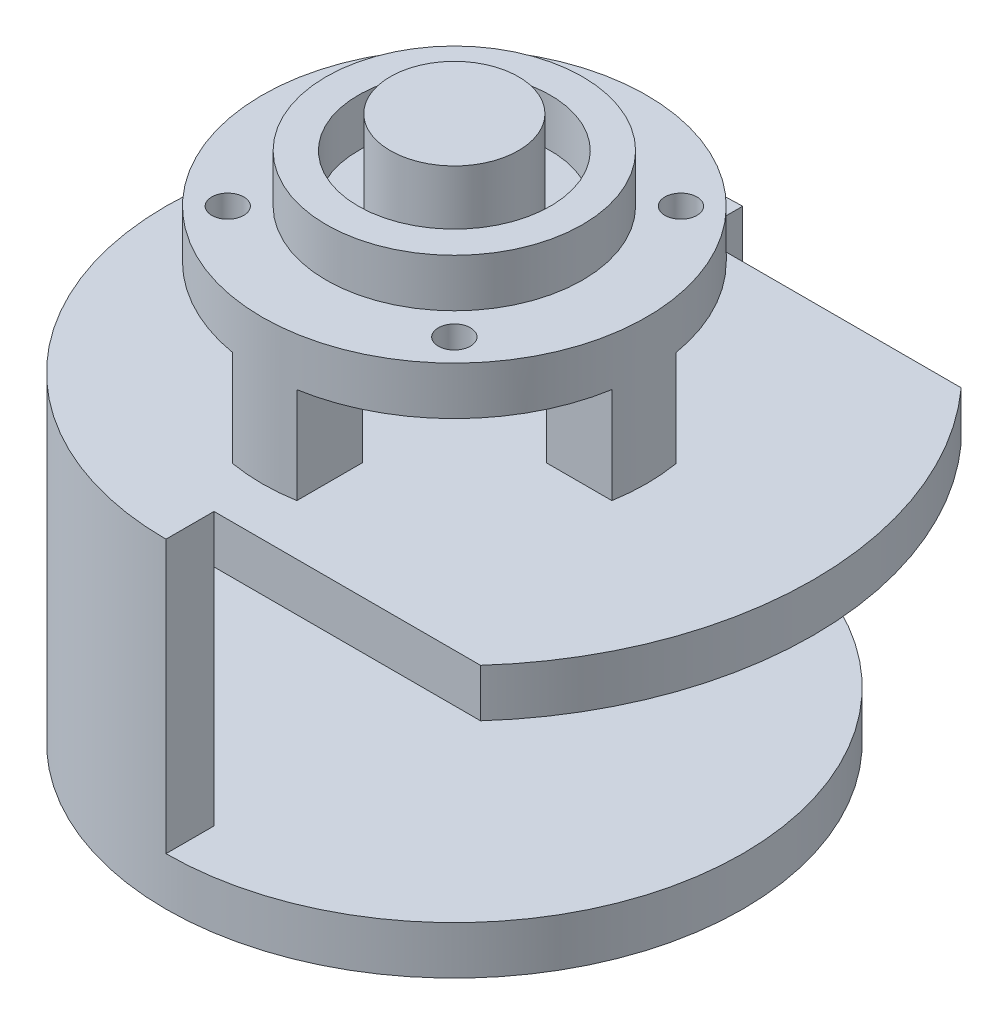
ISO-10303-21;
HEADER;
FILE_DESCRIPTION(('STEP AP214'),'2;1');
FILE_NAME('part.step','',(''),(''),'','','');
FILE_SCHEMA(('AUTOMOTIVE_DESIGN { 1 0 10303 214 1 1 1 1 }'));
ENDSEC;
DATA;
#1=APPLICATION_CONTEXT('core data for automotive mechanical design processes');
#2=APPLICATION_PROTOCOL_DEFINITION('international standard','automotive_design',2000,#1);
#3=PRODUCT_CONTEXT('',#1,'mechanical');
#4=PRODUCT('Part','Part','',(#3));
#5=PRODUCT_RELATED_PRODUCT_CATEGORY('part','',(#4));
#6=PRODUCT_DEFINITION_FORMATION('','',#4);
#7=PRODUCT_DEFINITION_CONTEXT('part definition',#1,'design');
#8=PRODUCT_DEFINITION('design','',#6,#7);
#9=PRODUCT_DEFINITION_SHAPE('','',#8);
#10=(LENGTH_UNIT() NAMED_UNIT(*) SI_UNIT(.MILLI.,.METRE.));
#11=(NAMED_UNIT(*) PLANE_ANGLE_UNIT() SI_UNIT($,.RADIAN.));
#12=(NAMED_UNIT(*) SI_UNIT($,.STERADIAN.) SOLID_ANGLE_UNIT());
#13=UNCERTAINTY_MEASURE_WITH_UNIT(LENGTH_MEASURE(1.E-05),#10,'distance_accuracy_value','');
#14=(GEOMETRIC_REPRESENTATION_CONTEXT(3) GLOBAL_UNCERTAINTY_ASSIGNED_CONTEXT((#13)) GLOBAL_UNIT_ASSIGNED_CONTEXT((#10,
#11,#12)) REPRESENTATION_CONTEXT('',''));
#15=CARTESIAN_POINT('',(0.,0.,0.));
#16=DIRECTION('',(0.,0.,1.));
#17=DIRECTION('',(1.,0.,0.));
#18=AXIS2_PLACEMENT_3D('',#15,#16,#17);
#19=CARTESIAN_POINT('',(0.,15.,0.));
#20=DIRECTION('',(0.,-1.,0.));
#21=DIRECTION('',(0.,0.,-1.));
#22=AXIS2_PLACEMENT_3D('',#19,#20,#21);
#23=CYLINDRICAL_SURFACE('',#22,90.);
#24=CARTESIAN_POINT('',(0.,15.,0.));
#25=DIRECTION('',(0.,1.,0.));
#26=DIRECTION('',(0.,0.,1.));
#27=AXIS2_PLACEMENT_3D('',#24,#25,#26);
#28=CIRCLE('',#27,90.);
#29=CARTESIAN_POINT('',(0.,15.,90.));
#30=VERTEX_POINT('',#29);
#31=CARTESIAN_POINT('',(0.,15.,-90.));
#32=VERTEX_POINT('',#31);
#33=EDGE_CURVE('E297',#30,#32,#28,.T.);
#34=ORIENTED_EDGE('',*,*,#33,.F.);
#35=DIRECTION('',(0.,-1.,0.));
#36=VECTOR('',#35,1.);
#37=CARTESIAN_POINT('',(0.,85.,90.));
#38=LINE('',#37,#36);
#39=CARTESIAN_POINT('',(0.,100.,90.));
#40=VERTEX_POINT('',#39);
#41=EDGE_CURVE('E298',#40,#30,#38,.T.);
#42=ORIENTED_EDGE('',*,*,#41,.F.);
#43=CARTESIAN_POINT('',(0.,100.,0.));
#44=DIRECTION('',(0.,1.,0.));
#45=DIRECTION('',(0.,0.,1.));
#46=AXIS2_PLACEMENT_3D('',#43,#44,#45);
#47=CIRCLE('',#46,90.);
#48=CARTESIAN_POINT('',(0.,100.,-90.));
#49=VERTEX_POINT('',#48);
#50=EDGE_CURVE('E242',#49,#40,#47,.T.);
#51=ORIENTED_EDGE('',*,*,#50,.F.);
#52=DIRECTION('',(0.,-1.,0.));
#53=VECTOR('',#52,1.);
#54=CARTESIAN_POINT('',(0.,85.,-90.));
#55=LINE('',#54,#53);
#56=EDGE_CURVE('E276',#49,#32,#55,.T.);
#57=ORIENTED_EDGE('',*,*,#56,.T.);
#58=EDGE_LOOP('',(#34,#42,#51,#57));
#59=FACE_BOUND('',#58,.T.);
#60=CARTESIAN_POINT('',(0.,0.,0.));
#61=DIRECTION('',(0.,1.,0.));
#62=DIRECTION('',(0.,0.,1.));
#63=AXIS2_PLACEMENT_3D('',#60,#61,#62);
#64=CIRCLE('',#63,90.);
#65=CARTESIAN_POINT('',(0.,0.,90.));
#66=VERTEX_POINT('',#65);
#67=EDGE_CURVE('E299',#66,#66,#64,.T.);
#68=ORIENTED_EDGE('',*,*,#67,.T.);
#69=EDGE_LOOP('',(#68));
#70=FACE_BOUND('',#69,.T.);
#71=ADVANCED_FACE('F50',(#59,#70),#23,.T.);
#72=CARTESIAN_POINT('',(0.,15.,0.));
#73=DIRECTION('',(0.,1.,0.));
#74=DIRECTION('',(0.,0.,1.));
#75=AXIS2_PLACEMENT_3D('',#72,#73,#74);
#76=PLANE('',#75);
#77=DIRECTION('',(0.,0.,-1.));
#78=VECTOR('',#77,1.);
#79=CARTESIAN_POINT('',(0.,15.,-75.));
#80=LINE('',#79,#78);
#81=CARTESIAN_POINT('',(0.,15.,-75.));
#82=VERTEX_POINT('',#81);
#83=EDGE_CURVE('E278',#82,#32,#80,.T.);
#84=ORIENTED_EDGE('',*,*,#83,.F.);
#85=CARTESIAN_POINT('',(0.,15.,0.));
#86=DIRECTION('',(0.,-1.,0.));
#87=DIRECTION('',(0.,0.,1.));
#88=AXIS2_PLACEMENT_3D('',#85,#86,#87);
#89=CIRCLE('',#88,75.);
#90=CARTESIAN_POINT('',(0.,15.,75.));
#91=VERTEX_POINT('',#90);
#92=EDGE_CURVE('E281',#91,#82,#89,.T.);
#93=ORIENTED_EDGE('',*,*,#92,.F.);
#94=DIRECTION('',(0.,0.,-1.));
#95=VECTOR('',#94,1.);
#96=CARTESIAN_POINT('',(0.,15.,90.));
#97=LINE('',#96,#95);
#98=EDGE_CURVE('E274',#30,#91,#97,.T.);
#99=ORIENTED_EDGE('',*,*,#98,.F.);
#100=ORIENTED_EDGE('',*,*,#33,.T.);
#101=EDGE_LOOP('',(#84,#93,#99,#100));
#102=FACE_BOUND('',#101,.T.);
#103=ADVANCED_FACE('F437',(#102),#76,.T.);
#104=CARTESIAN_POINT('',(0.,0.,0.));
#105=DIRECTION('',(0.,1.,0.));
#106=DIRECTION('',(0.,0.,1.));
#107=AXIS2_PLACEMENT_3D('',#104,#105,#106);
#108=PLANE('',#107);
#109=ORIENTED_EDGE('',*,*,#67,.F.);
#110=EDGE_LOOP('',(#109));
#111=FACE_BOUND('',#110,.T.);
#112=ADVANCED_FACE('F443',(#111),#108,.F.);
#113=CARTESIAN_POINT('',(0.,85.,90.));
#114=DIRECTION('',(-1.,0.,0.));
#115=DIRECTION('',(0.,0.,1.));
#116=AXIS2_PLACEMENT_3D('',#113,#114,#115);
#117=PLANE('',#116);
#118=ORIENTED_EDGE('',*,*,#98,.T.);
#119=DIRECTION('',(0.,-1.,0.));
#120=VECTOR('',#119,1.);
#121=CARTESIAN_POINT('',(0.,85.,75.));
#122=LINE('',#121,#120);
#123=CARTESIAN_POINT('',(0.,85.,75.));
#124=VERTEX_POINT('',#123);
#125=EDGE_CURVE('E291',#124,#91,#122,.T.);
#126=ORIENTED_EDGE('',*,*,#125,.F.);
#127=DIRECTION('',(0.,-1.,0.));
#128=VECTOR('',#127,1.);
#129=CARTESIAN_POINT('',(0.,100.,75.));
#130=LINE('',#129,#128);
#131=CARTESIAN_POINT('',(0.,100.,75.));
#132=VERTEX_POINT('',#131);
#133=EDGE_CURVE('E275',#132,#124,#130,.T.);
#134=ORIENTED_EDGE('',*,*,#133,.F.);
#135=DIRECTION('',(0.,0.,-1.));
#136=VECTOR('',#135,1.);
#137=CARTESIAN_POINT('',(0.,100.,0.));
#138=LINE('',#137,#136);
#139=EDGE_CURVE('E248',#40,#132,#138,.T.);
#140=ORIENTED_EDGE('',*,*,#139,.F.);
#141=ORIENTED_EDGE('',*,*,#41,.T.);
#142=EDGE_LOOP('',(#118,#126,#134,#140,#141));
#143=FACE_BOUND('',#142,.T.);
#144=ADVANCED_FACE('F454',(#143),#117,.F.);
#145=CARTESIAN_POINT('',(0.,85.,0.));
#146=DIRECTION('',(0.,-1.,0.));
#147=DIRECTION('',(0.,0.,-1.));
#148=AXIS2_PLACEMENT_3D('',#145,#146,#147);
#149=CYLINDRICAL_SURFACE('',#148,75.);
#150=ORIENTED_EDGE('',*,*,#92,.T.);
#151=DIRECTION('',(0.,-1.,0.));
#152=VECTOR('',#151,1.);
#153=CARTESIAN_POINT('',(0.,85.,-75.));
#154=LINE('',#153,#152);
#155=CARTESIAN_POINT('',(0.,85.,-75.));
#156=VERTEX_POINT('',#155);
#157=EDGE_CURVE('E290',#156,#82,#154,.T.);
#158=ORIENTED_EDGE('',*,*,#157,.F.);
#159=CARTESIAN_POINT('',(0.,85.,0.));
#160=DIRECTION('',(0.,-1.,0.));
#161=DIRECTION('',(0.,0.,1.));
#162=AXIS2_PLACEMENT_3D('',#159,#160,#161);
#163=CIRCLE('',#162,75.);
#164=EDGE_CURVE('E277',#124,#156,#163,.T.);
#165=ORIENTED_EDGE('',*,*,#164,.F.);
#166=ORIENTED_EDGE('',*,*,#125,.T.);
#167=EDGE_LOOP('',(#150,#158,#165,#166));
#168=FACE_BOUND('',#167,.T.);
#169=ADVANCED_FACE('F457',(#168),#149,.F.);
#170=CARTESIAN_POINT('',(0.,85.,-75.));
#171=DIRECTION('',(-1.,0.,0.));
#172=DIRECTION('',(0.,0.,1.));
#173=AXIS2_PLACEMENT_3D('',#170,#171,#172);
#174=PLANE('',#173);
#175=ORIENTED_EDGE('',*,*,#83,.T.);
#176=ORIENTED_EDGE('',*,*,#56,.F.);
#177=DIRECTION('',(0.,0.,-1.));
#178=VECTOR('',#177,1.);
#179=CARTESIAN_POINT('',(0.,100.,0.));
#180=LINE('',#179,#178);
#181=CARTESIAN_POINT('',(0.,100.,-75.));
#182=VERTEX_POINT('',#181);
#183=EDGE_CURVE('E245',#182,#49,#180,.T.);
#184=ORIENTED_EDGE('',*,*,#183,.F.);
#185=DIRECTION('',(0.,-1.,0.));
#186=VECTOR('',#185,1.);
#187=CARTESIAN_POINT('',(0.,100.,-75.));
#188=LINE('',#187,#186);
#189=EDGE_CURVE('E256',#182,#156,#188,.T.);
#190=ORIENTED_EDGE('',*,*,#189,.T.);
#191=ORIENTED_EDGE('',*,*,#157,.T.);
#192=EDGE_LOOP('',(#175,#176,#184,#190,#191));
#193=FACE_BOUND('',#192,.T.);
#194=ADVANCED_FACE('F465',(#193),#174,.F.);
#195=CARTESIAN_POINT('',(0.,85.,0.));
#196=DIRECTION('',(0.,1.,0.));
#197=DIRECTION('',(0.,0.,1.));
#198=AXIS2_PLACEMENT_3D('',#195,#196,#197);
#199=PLANE('',#198);
#200=DIRECTION('',(1.,0.,0.));
#201=VECTOR('',#200,1.);
#202=CARTESIAN_POINT('',(0.,85.,75.));
#203=LINE('',#202,#201);
#204=CARTESIAN_POINT('',(83.18052656722,85.,75.));
#205=VERTEX_POINT('',#204);
#206=EDGE_CURVE('E233',#124,#205,#203,.T.);
#207=ORIENTED_EDGE('',*,*,#206,.F.);
#208=ORIENTED_EDGE('',*,*,#164,.T.);
#209=DIRECTION('',(1.,0.,0.));
#210=VECTOR('',#209,1.);
#211=CARTESIAN_POINT('',(0.,85.,-75.));
#212=LINE('',#211,#210);
#213=CARTESIAN_POINT('',(83.18052656722,85.,-75.));
#214=VERTEX_POINT('',#213);
#215=EDGE_CURVE('E246',#156,#214,#212,.T.);
#216=ORIENTED_EDGE('',*,*,#215,.T.);
#217=CARTESIAN_POINT('',(0.,85.,0.));
#218=DIRECTION('',(0.,1.,0.));
#219=DIRECTION('',(0.,0.,1.));
#220=AXIS2_PLACEMENT_3D('',#217,#218,#219);
#221=CIRCLE('',#220,112.);
#222=EDGE_CURVE('E257',#205,#214,#221,.T.);
#223=ORIENTED_EDGE('',*,*,#222,.F.);
#224=EDGE_LOOP('',(#207,#208,#216,#223));
#225=FACE_BOUND('',#224,.T.);
#226=ADVANCED_FACE('F466',(#225),#199,.F.);
#227=CARTESIAN_POINT('',(0.,100.,75.));
#228=DIRECTION('',(0.,0.,-1.));
#229=DIRECTION('',(-1.,0.,0.));
#230=AXIS2_PLACEMENT_3D('',#227,#228,#229);
#231=PLANE('',#230);
#232=ORIENTED_EDGE('',*,*,#206,.T.);
#233=DIRECTION('',(0.,-1.,0.));
#234=VECTOR('',#233,1.);
#235=CARTESIAN_POINT('',(83.18052656722,100.,75.));
#236=LINE('',#235,#234);
#237=CARTESIAN_POINT('',(83.18052656722,100.,75.));
#238=VERTEX_POINT('',#237);
#239=EDGE_CURVE('E267',#238,#205,#236,.T.);
#240=ORIENTED_EDGE('',*,*,#239,.F.);
#241=DIRECTION('',(1.,0.,0.));
#242=VECTOR('',#241,1.);
#243=CARTESIAN_POINT('',(0.,100.,75.));
#244=LINE('',#243,#242);
#245=EDGE_CURVE('E253',#132,#238,#244,.T.);
#246=ORIENTED_EDGE('',*,*,#245,.F.);
#247=ORIENTED_EDGE('',*,*,#133,.T.);
#248=EDGE_LOOP('',(#232,#240,#246,#247));
#249=FACE_BOUND('',#248,.T.);
#250=ADVANCED_FACE('F469',(#249),#231,.F.);
#251=CARTESIAN_POINT('',(0.,100.,0.));
#252=DIRECTION('',(0.,-1.,0.));
#253=DIRECTION('',(0.,0.,-1.));
#254=AXIS2_PLACEMENT_3D('',#251,#252,#253);
#255=CYLINDRICAL_SURFACE('',#254,112.);
#256=ORIENTED_EDGE('',*,*,#222,.T.);
#257=DIRECTION('',(0.,-1.,0.));
#258=VECTOR('',#257,1.);
#259=CARTESIAN_POINT('',(83.18052656722,100.,-75.));
#260=LINE('',#259,#258);
#261=CARTESIAN_POINT('',(83.18052656722,100.,-75.));
#262=VERTEX_POINT('',#261);
#263=EDGE_CURVE('E270',#262,#214,#260,.T.);
#264=ORIENTED_EDGE('',*,*,#263,.F.);
#265=CARTESIAN_POINT('',(0.,100.,0.));
#266=DIRECTION('',(0.,1.,0.));
#267=DIRECTION('',(0.,0.,1.));
#268=AXIS2_PLACEMENT_3D('',#265,#266,#267);
#269=CIRCLE('',#268,112.);
#270=EDGE_CURVE('E251',#238,#262,#269,.T.);
#271=ORIENTED_EDGE('',*,*,#270,.F.);
#272=ORIENTED_EDGE('',*,*,#239,.T.);
#273=EDGE_LOOP('',(#256,#264,#271,#272));
#274=FACE_BOUND('',#273,.T.);
#275=ADVANCED_FACE('F473',(#274),#255,.T.);
#276=CARTESIAN_POINT('',(0.,100.,-75.));
#277=DIRECTION('',(0.,0.,-1.));
#278=DIRECTION('',(-1.,0.,0.));
#279=AXIS2_PLACEMENT_3D('',#276,#277,#278);
#280=PLANE('',#279);
#281=ORIENTED_EDGE('',*,*,#215,.F.);
#282=ORIENTED_EDGE('',*,*,#189,.F.);
#283=DIRECTION('',(1.,0.,0.));
#284=VECTOR('',#283,1.);
#285=CARTESIAN_POINT('',(0.,100.,-75.));
#286=LINE('',#285,#284);
#287=EDGE_CURVE('E254',#182,#262,#286,.T.);
#288=ORIENTED_EDGE('',*,*,#287,.T.);
#289=ORIENTED_EDGE('',*,*,#263,.T.);
#290=EDGE_LOOP('',(#281,#282,#288,#289));
#291=FACE_BOUND('',#290,.T.);
#292=ADVANCED_FACE('F474',(#291),#280,.T.);
#293=CARTESIAN_POINT('',(0.,100.,0.));
#294=DIRECTION('',(0.,1.,0.));
#295=DIRECTION('',(0.,0.,1.));
#296=AXIS2_PLACEMENT_3D('',#293,#294,#295);
#297=PLANE('',#296);
#298=CARTESIAN_POINT('',(0.,100.,0.));
#299=DIRECTION('',(0.,1.,0.));
#300=DIRECTION('',(0.,0.,1.));
#301=AXIS2_PLACEMENT_3D('',#298,#299,#300);
#302=CIRCLE('',#301,60.);
#303=CARTESIAN_POINT('',(-10.,100.,59.1607978309962));
#304=VERTEX_POINT('',#303);
#305=CARTESIAN_POINT('',(9.99999999999999,100.,59.1607978309962));
#306=VERTEX_POINT('',#305);
#307=EDGE_CURVE('E235',#304,#306,#302,.T.);
#308=ORIENTED_EDGE('',*,*,#307,.F.);
#309=DIRECTION('',(0.,0.,-1.));
#310=VECTOR('',#309,1.);
#311=CARTESIAN_POINT('',(-10.,100.,59.1607978309962));
#312=LINE('',#311,#310);
#313=CARTESIAN_POINT('',(-10.,100.,38.7298334620742));
#314=VERTEX_POINT('',#313);
#315=EDGE_CURVE('E380',#304,#314,#312,.T.);
#316=ORIENTED_EDGE('',*,*,#315,.T.);
#317=CARTESIAN_POINT('',(0.,100.,0.));
#318=DIRECTION('',(0.,1.,0.));
#319=DIRECTION('',(0.,0.,1.));
#320=AXIS2_PLACEMENT_3D('',#317,#318,#319);
#321=CIRCLE('',#320,40.);
#322=CARTESIAN_POINT('',(9.99999999999998,100.,38.7298334620742));
#323=VERTEX_POINT('',#322);
#324=EDGE_CURVE('E302',#323,#314,#321,.F.);
#325=ORIENTED_EDGE('',*,*,#324,.F.);
#326=DIRECTION('',(0.,0.,1.));
#327=VECTOR('',#326,1.);
#328=CARTESIAN_POINT('',(9.99999999999999,100.,59.1607978309962));
#329=LINE('',#328,#327);
#330=EDGE_CURVE('E392',#323,#306,#329,.T.);
#331=ORIENTED_EDGE('',*,*,#330,.T.);
#332=EDGE_LOOP('',(#308,#316,#325,#331));
#333=FACE_BOUND('',#332,.T.);
#334=CARTESIAN_POINT('',(59.1607978309962,100.,10.));
#335=VERTEX_POINT('',#334);
#336=CARTESIAN_POINT('',(59.1607978309962,100.,-9.99999999999998));
#337=VERTEX_POINT('',#336);
#338=EDGE_CURVE('E227',#335,#337,#302,.T.);
#339=ORIENTED_EDGE('',*,*,#338,.F.);
#340=DIRECTION('',(-1.,0.,0.));
#341=VECTOR('',#340,1.);
#342=CARTESIAN_POINT('',(59.1607978309962,100.,10.));
#343=LINE('',#342,#341);
#344=CARTESIAN_POINT('',(38.7298334620742,100.,10.));
#345=VERTEX_POINT('',#344);
#346=EDGE_CURVE('E399',#335,#345,#343,.T.);
#347=ORIENTED_EDGE('',*,*,#346,.T.);
#348=CARTESIAN_POINT('',(38.7298334620742,100.,-9.99999999999998));
#349=VERTEX_POINT('',#348);
#350=EDGE_CURVE('E305',#349,#345,#321,.F.);
#351=ORIENTED_EDGE('',*,*,#350,.F.);
#352=DIRECTION('',(1.,0.,0.));
#353=VECTOR('',#352,1.);
#354=CARTESIAN_POINT('',(59.1607978309962,100.,-9.99999999999998));
#355=LINE('',#354,#353);
#356=EDGE_CURVE('E213',#349,#337,#355,.T.);
#357=ORIENTED_EDGE('',*,*,#356,.T.);
#358=EDGE_LOOP('',(#339,#347,#351,#357));
#359=FACE_BOUND('',#358,.T.);
#360=CARTESIAN_POINT('',(10.,100.,-59.1607978309962));
#361=VERTEX_POINT('',#360);
#362=CARTESIAN_POINT('',(-10.,100.,-59.1607978309962));
#363=VERTEX_POINT('',#362);
#364=EDGE_CURVE('E225',#361,#363,#302,.T.);
#365=ORIENTED_EDGE('',*,*,#364,.F.);
#366=DIRECTION('',(0.,0.,1.));
#367=VECTOR('',#366,1.);
#368=CARTESIAN_POINT('',(10.,100.,-59.1607978309962));
#369=LINE('',#368,#367);
#370=CARTESIAN_POINT('',(10.,100.,-38.7298334620742));
#371=VERTEX_POINT('',#370);
#372=EDGE_CURVE('E203',#361,#371,#369,.T.);
#373=ORIENTED_EDGE('',*,*,#372,.T.);
#374=CARTESIAN_POINT('',(-10.,100.,-38.7298334620742));
#375=VERTEX_POINT('',#374);
#376=EDGE_CURVE('E313',#375,#371,#321,.F.);
#377=ORIENTED_EDGE('',*,*,#376,.F.);
#378=DIRECTION('',(0.,0.,-1.));
#379=VECTOR('',#378,1.);
#380=CARTESIAN_POINT('',(-10.,100.,-59.1607978309962));
#381=LINE('',#380,#379);
#382=EDGE_CURVE('E229',#375,#363,#381,.T.);
#383=ORIENTED_EDGE('',*,*,#382,.T.);
#384=EDGE_LOOP('',(#365,#373,#377,#383));
#385=FACE_BOUND('',#384,.T.);
#386=DIRECTION('',(-1.,0.,0.));
#387=VECTOR('',#386,1.);
#388=CARTESIAN_POINT('',(-59.1607978309962,100.,9.99999999999999));
#389=LINE('',#388,#387);
#390=CARTESIAN_POINT('',(-38.7298334620742,100.,9.99999999999997));
#391=VERTEX_POINT('',#390);
#392=CARTESIAN_POINT('',(-59.1607978309962,100.,9.99999999999999));
#393=VERTEX_POINT('',#392);
#394=EDGE_CURVE('E356',#391,#393,#389,.T.);
#395=ORIENTED_EDGE('',*,*,#394,.T.);
#396=CARTESIAN_POINT('',(-59.1607978309962,100.,-10.));
#397=VERTEX_POINT('',#396);
#398=EDGE_CURVE('E231',#397,#393,#302,.T.);
#399=ORIENTED_EDGE('',*,*,#398,.F.);
#400=DIRECTION('',(1.,0.,0.));
#401=VECTOR('',#400,1.);
#402=CARTESIAN_POINT('',(-59.1607978309962,100.,-10.));
#403=LINE('',#402,#401);
#404=CARTESIAN_POINT('',(-38.7298334620742,100.,-10.));
#405=VERTEX_POINT('',#404);
#406=EDGE_CURVE('E340',#397,#405,#403,.T.);
#407=ORIENTED_EDGE('',*,*,#406,.T.);
#408=EDGE_CURVE('E53',#391,#405,#321,.F.);
#409=ORIENTED_EDGE('',*,*,#408,.F.);
#410=EDGE_LOOP('',(#395,#399,#407,#409));
#411=FACE_BOUND('',#410,.T.);
#412=ORIENTED_EDGE('',*,*,#183,.T.);
#413=ORIENTED_EDGE('',*,*,#50,.T.);
#414=ORIENTED_EDGE('',*,*,#139,.T.);
#415=ORIENTED_EDGE('',*,*,#245,.T.);
#416=ORIENTED_EDGE('',*,*,#270,.T.);
#417=ORIENTED_EDGE('',*,*,#287,.F.);
#418=EDGE_LOOP('',(#412,#413,#414,#415,#416,#417));
#419=FACE_BOUND('',#418,.T.);
#420=ADVANCED_FACE('F230',(#333,#359,#385,#411,#419),#297,.T.);
#421=CARTESIAN_POINT('',(0.,140.,0.));
#422=DIRECTION('',(0.,-1.,0.));
#423=DIRECTION('',(0.,0.,-1.));
#424=AXIS2_PLACEMENT_3D('',#421,#422,#423);
#425=CYLINDRICAL_SURFACE('',#424,60.);
#426=ORIENTED_EDGE('',*,*,#398,.T.);
#427=DIRECTION('',(0.,1.,0.));
#428=VECTOR('',#427,1.);
#429=CARTESIAN_POINT('',(-59.1607978309962,100.,9.99999999999999));
#430=LINE('',#429,#428);
#431=CARTESIAN_POINT('',(-59.1607978309962,130.,9.99999999999999));
#432=VERTEX_POINT('',#431);
#433=EDGE_CURVE('E358',#393,#432,#430,.T.);
#434=ORIENTED_EDGE('',*,*,#433,.T.);
#435=CARTESIAN_POINT('',(0.,130.,0.));
#436=DIRECTION('',(0.,1.,0.));
#437=DIRECTION('',(0.,0.,1.));
#438=AXIS2_PLACEMENT_3D('',#435,#436,#437);
#439=CIRCLE('',#438,60.);
#440=CARTESIAN_POINT('',(-10.,130.,59.1607978309962));
#441=VERTEX_POINT('',#440);
#442=EDGE_CURVE('E363',#432,#441,#439,.T.);
#443=ORIENTED_EDGE('',*,*,#442,.T.);
#444=DIRECTION('',(0.,1.,0.));
#445=VECTOR('',#444,1.);
#446=CARTESIAN_POINT('',(-10.,100.,59.1607978309962));
#447=LINE('',#446,#445);
#448=EDGE_CURVE('E374',#304,#441,#447,.T.);
#449=ORIENTED_EDGE('',*,*,#448,.F.);
#450=ORIENTED_EDGE('',*,*,#307,.T.);
#451=DIRECTION('',(0.,1.,0.));
#452=VECTOR('',#451,1.);
#453=CARTESIAN_POINT('',(9.99999999999999,100.,59.1607978309962));
#454=LINE('',#453,#452);
#455=CARTESIAN_POINT('',(9.99999999999999,130.,59.1607978309962));
#456=VERTEX_POINT('',#455);
#457=EDGE_CURVE('E407',#306,#456,#454,.T.);
#458=ORIENTED_EDGE('',*,*,#457,.T.);
#459=CARTESIAN_POINT('',(0.,130.,0.));
#460=DIRECTION('',(0.,1.,0.));
#461=DIRECTION('',(0.,0.,1.));
#462=AXIS2_PLACEMENT_3D('',#459,#460,#461);
#463=CIRCLE('',#462,60.);
#464=CARTESIAN_POINT('',(59.1607978309962,130.,10.));
#465=VERTEX_POINT('',#464);
#466=EDGE_CURVE('E365',#456,#465,#463,.T.);
#467=ORIENTED_EDGE('',*,*,#466,.T.);
#468=DIRECTION('',(0.,1.,0.));
#469=VECTOR('',#468,1.);
#470=CARTESIAN_POINT('',(59.1607978309962,100.,10.));
#471=LINE('',#470,#469);
#472=EDGE_CURVE('E397',#335,#465,#471,.T.);
#473=ORIENTED_EDGE('',*,*,#472,.F.);
#474=ORIENTED_EDGE('',*,*,#338,.T.);
#475=DIRECTION('',(0.,1.,0.));
#476=VECTOR('',#475,1.);
#477=CARTESIAN_POINT('',(59.1607978309962,100.,-9.99999999999998));
#478=LINE('',#477,#476);
#479=CARTESIAN_POINT('',(59.1607978309962,130.,-9.99999999999998));
#480=VERTEX_POINT('',#479);
#481=EDGE_CURVE('E347',#337,#480,#478,.T.);
#482=ORIENTED_EDGE('',*,*,#481,.T.);
#483=CARTESIAN_POINT('',(0.,130.,0.));
#484=DIRECTION('',(0.,1.,0.));
#485=DIRECTION('',(0.,0.,1.));
#486=AXIS2_PLACEMENT_3D('',#483,#484,#485);
#487=CIRCLE('',#486,60.);
#488=CARTESIAN_POINT('',(10.,130.,-59.1607978309962));
#489=VERTEX_POINT('',#488);
#490=EDGE_CURVE('E221',#480,#489,#487,.T.);
#491=ORIENTED_EDGE('',*,*,#490,.T.);
#492=DIRECTION('',(0.,1.,0.));
#493=VECTOR('',#492,1.);
#494=CARTESIAN_POINT('',(10.,100.,-59.1607978309962));
#495=LINE('',#494,#493);
#496=EDGE_CURVE('E202',#361,#489,#495,.T.);
#497=ORIENTED_EDGE('',*,*,#496,.F.);
#498=ORIENTED_EDGE('',*,*,#364,.T.);
#499=DIRECTION('',(0.,1.,0.));
#500=VECTOR('',#499,1.);
#501=CARTESIAN_POINT('',(-10.,100.,-59.1607978309962));
#502=LINE('',#501,#500);
#503=CARTESIAN_POINT('',(-10.,130.,-59.1607978309962));
#504=VERTEX_POINT('',#503);
#505=EDGE_CURVE('E239',#363,#504,#502,.T.);
#506=ORIENTED_EDGE('',*,*,#505,.T.);
#507=CARTESIAN_POINT('',(0.,130.,0.));
#508=DIRECTION('',(0.,1.,0.));
#509=DIRECTION('',(0.,0.,1.));
#510=AXIS2_PLACEMENT_3D('',#507,#508,#509);
#511=CIRCLE('',#510,60.);
#512=CARTESIAN_POINT('',(-59.1607978309962,130.,-10.));
#513=VERTEX_POINT('',#512);
#514=EDGE_CURVE('E344',#504,#513,#511,.T.);
#515=ORIENTED_EDGE('',*,*,#514,.T.);
#516=DIRECTION('',(0.,1.,0.));
#517=VECTOR('',#516,1.);
#518=CARTESIAN_POINT('',(-59.1607978309962,100.,-10.));
#519=LINE('',#518,#517);
#520=EDGE_CURVE('E328',#397,#513,#519,.T.);
#521=ORIENTED_EDGE('',*,*,#520,.F.);
#522=EDGE_LOOP('',(#426,#434,#443,#449,#450,#458,#467,#473,#474,#482,#491,#497,#498,#506,#515,#521));
#523=FACE_BOUND('',#522,.T.);
#524=CARTESIAN_POINT('',(0.,145.,0.));
#525=DIRECTION('',(0.,1.,0.));
#526=DIRECTION('',(0.,0.,1.));
#527=AXIS2_PLACEMENT_3D('',#524,#525,#526);
#528=CIRCLE('',#527,60.);
#529=CARTESIAN_POINT('',(0.,145.,60.));
#530=VERTEX_POINT('',#529);
#531=EDGE_CURVE('E517',#530,#530,#528,.T.);
#532=ORIENTED_EDGE('',*,*,#531,.F.);
#533=EDGE_LOOP('',(#532));
#534=FACE_BOUND('',#533,.T.);
#535=ADVANCED_FACE('F218',(#523,#534),#425,.T.);
#536=CARTESIAN_POINT('',(0.,140.,0.));
#537=DIRECTION('',(0.,-1.,0.));
#538=DIRECTION('',(0.,0.,-1.));
#539=AXIS2_PLACEMENT_3D('',#536,#537,#538);
#540=CYLINDRICAL_SURFACE('',#539,40.);
#541=DIRECTION('',(0.,1.,0.));
#542=VECTOR('',#541,1.);
#543=CARTESIAN_POINT('',(-38.7298334620742,100.,9.99999999999997));
#544=LINE('',#543,#542);
#545=CARTESIAN_POINT('',(-38.7298334620742,130.,9.99999999999997));
#546=VERTEX_POINT('',#545);
#547=EDGE_CURVE('E364',#391,#546,#544,.T.);
#548=ORIENTED_EDGE('',*,*,#547,.F.);
#549=ORIENTED_EDGE('',*,*,#408,.T.);
#550=DIRECTION('',(0.,1.,0.));
#551=VECTOR('',#550,1.);
#552=CARTESIAN_POINT('',(-38.7298334620742,100.,-10.));
#553=LINE('',#552,#551);
#554=CARTESIAN_POINT('',(-38.7298334620742,130.,-10.));
#555=VERTEX_POINT('',#554);
#556=EDGE_CURVE('E326',#405,#555,#553,.T.);
#557=ORIENTED_EDGE('',*,*,#556,.T.);
#558=CARTESIAN_POINT('',(0.,130.,0.));
#559=DIRECTION('',(0.,-1.,0.));
#560=DIRECTION('',(0.,0.,1.));
#561=AXIS2_PLACEMENT_3D('',#558,#559,#560);
#562=CIRCLE('',#561,40.);
#563=CARTESIAN_POINT('',(-10.,130.,-38.7298334620742));
#564=VERTEX_POINT('',#563);
#565=EDGE_CURVE('E325',#555,#564,#562,.T.);
#566=ORIENTED_EDGE('',*,*,#565,.T.);
#567=DIRECTION('',(0.,1.,0.));
#568=VECTOR('',#567,1.);
#569=CARTESIAN_POINT('',(-10.,100.,-38.7298334620742));
#570=LINE('',#569,#568);
#571=EDGE_CURVE('E321',#375,#564,#570,.T.);
#572=ORIENTED_EDGE('',*,*,#571,.F.);
#573=ORIENTED_EDGE('',*,*,#376,.T.);
#574=DIRECTION('',(0.,1.,0.));
#575=VECTOR('',#574,1.);
#576=CARTESIAN_POINT('',(10.,100.,-38.7298334620742));
#577=LINE('',#576,#575);
#578=CARTESIAN_POINT('',(10.,130.,-38.7298334620742));
#579=VERTEX_POINT('',#578);
#580=EDGE_CURVE('E208',#371,#579,#577,.T.);
#581=ORIENTED_EDGE('',*,*,#580,.T.);
#582=CARTESIAN_POINT('',(0.,130.,0.));
#583=DIRECTION('',(0.,-1.,0.));
#584=DIRECTION('',(0.,0.,1.));
#585=AXIS2_PLACEMENT_3D('',#582,#583,#584);
#586=CIRCLE('',#585,40.);
#587=CARTESIAN_POINT('',(38.7298334620742,130.,-9.99999999999998));
#588=VERTEX_POINT('',#587);
#589=EDGE_CURVE('E534',#579,#588,#586,.T.);
#590=ORIENTED_EDGE('',*,*,#589,.T.);
#591=DIRECTION('',(0.,1.,0.));
#592=VECTOR('',#591,1.);
#593=CARTESIAN_POINT('',(38.7298334620742,100.,-9.99999999999998));
#594=LINE('',#593,#592);
#595=EDGE_CURVE('E537',#349,#588,#594,.T.);
#596=ORIENTED_EDGE('',*,*,#595,.F.);
#597=ORIENTED_EDGE('',*,*,#350,.T.);
#598=DIRECTION('',(0.,1.,0.));
#599=VECTOR('',#598,1.);
#600=CARTESIAN_POINT('',(38.7298334620742,100.,10.));
#601=LINE('',#600,#599);
#602=CARTESIAN_POINT('',(38.7298334620742,130.,10.));
#603=VERTEX_POINT('',#602);
#604=EDGE_CURVE('E400',#345,#603,#601,.T.);
#605=ORIENTED_EDGE('',*,*,#604,.T.);
#606=CARTESIAN_POINT('',(0.,130.,0.));
#607=DIRECTION('',(0.,-1.,0.));
#608=DIRECTION('',(0.,0.,1.));
#609=AXIS2_PLACEMENT_3D('',#606,#607,#608);
#610=CIRCLE('',#609,40.);
#611=CARTESIAN_POINT('',(9.99999999999998,130.,38.7298334620742));
#612=VERTEX_POINT('',#611);
#613=EDGE_CURVE('E403',#603,#612,#610,.T.);
#614=ORIENTED_EDGE('',*,*,#613,.T.);
#615=DIRECTION('',(0.,1.,0.));
#616=VECTOR('',#615,1.);
#617=CARTESIAN_POINT('',(9.99999999999998,100.,38.7298334620742));
#618=LINE('',#617,#616);
#619=EDGE_CURVE('E412',#323,#612,#618,.T.);
#620=ORIENTED_EDGE('',*,*,#619,.F.);
#621=ORIENTED_EDGE('',*,*,#324,.T.);
#622=DIRECTION('',(0.,1.,0.));
#623=VECTOR('',#622,1.);
#624=CARTESIAN_POINT('',(-10.,100.,38.7298334620742));
#625=LINE('',#624,#623);
#626=CARTESIAN_POINT('',(-10.,130.,38.7298334620742));
#627=VERTEX_POINT('',#626);
#628=EDGE_CURVE('E369',#314,#627,#625,.T.);
#629=ORIENTED_EDGE('',*,*,#628,.T.);
#630=CARTESIAN_POINT('',(0.,130.,0.));
#631=DIRECTION('',(0.,-1.,0.));
#632=DIRECTION('',(0.,0.,1.));
#633=AXIS2_PLACEMENT_3D('',#630,#631,#632);
#634=CIRCLE('',#633,40.);
#635=EDGE_CURVE('E382',#627,#546,#634,.T.);
#636=ORIENTED_EDGE('',*,*,#635,.T.);
#637=EDGE_LOOP('',(#548,#549,#557,#566,#572,#573,#581,#590,#596,#597,#605,#614,#620,#621,#629,#636));
#638=FACE_BOUND('',#637,.T.);
#639=CARTESIAN_POINT('',(0.,140.,0.));
#640=DIRECTION('',(0.,1.,0.));
#641=DIRECTION('',(0.,0.,1.));
#642=AXIS2_PLACEMENT_3D('',#639,#640,#641);
#643=CIRCLE('',#642,40.);
#644=CARTESIAN_POINT('',(0.,140.,40.));
#645=VERTEX_POINT('',#644);
#646=EDGE_CURVE('E238',#645,#645,#643,.T.);
#647=ORIENTED_EDGE('',*,*,#646,.T.);
#648=EDGE_LOOP('',(#647));
#649=FACE_BOUND('',#648,.T.);
#650=ADVANCED_FACE('F320',(#638,#649),#540,.F.);
#651=CARTESIAN_POINT('',(-10.,100.,-59.1607978309962));
#652=DIRECTION('',(1.,0.,0.));
#653=DIRECTION('',(0.,0.,-1.));
#654=AXIS2_PLACEMENT_3D('',#651,#652,#653);
#655=PLANE('',#654);
#656=DIRECTION('',(0.,0.,-1.));
#657=VECTOR('',#656,1.);
#658=CARTESIAN_POINT('',(-10.,130.,-59.1607978309962));
#659=LINE('',#658,#657);
#660=EDGE_CURVE('E339',#564,#504,#659,.T.);
#661=ORIENTED_EDGE('',*,*,#660,.T.);
#662=ORIENTED_EDGE('',*,*,#505,.F.);
#663=ORIENTED_EDGE('',*,*,#382,.F.);
#664=ORIENTED_EDGE('',*,*,#571,.T.);
#665=EDGE_LOOP('',(#661,#662,#663,#664));
#666=FACE_BOUND('',#665,.T.);
#667=ADVANCED_FACE('F346',(#666),#655,.F.);
#668=CARTESIAN_POINT('',(-59.1607978309962,100.,-10.));
#669=DIRECTION('',(0.,0.,1.));
#670=DIRECTION('',(1.,0.,0.));
#671=AXIS2_PLACEMENT_3D('',#668,#669,#670);
#672=PLANE('',#671);
#673=DIRECTION('',(1.,0.,0.));
#674=VECTOR('',#673,1.);
#675=CARTESIAN_POINT('',(-59.1607978309962,130.,-10.));
#676=LINE('',#675,#674);
#677=EDGE_CURVE('E345',#513,#555,#676,.T.);
#678=ORIENTED_EDGE('',*,*,#677,.T.);
#679=ORIENTED_EDGE('',*,*,#556,.F.);
#680=ORIENTED_EDGE('',*,*,#406,.F.);
#681=ORIENTED_EDGE('',*,*,#520,.T.);
#682=EDGE_LOOP('',(#678,#679,#680,#681));
#683=FACE_BOUND('',#682,.T.);
#684=ADVANCED_FACE('F351',(#683),#672,.F.);
#685=CARTESIAN_POINT('',(0.,130.,0.));
#686=DIRECTION('',(0.,1.,0.));
#687=DIRECTION('',(0.,0.,1.));
#688=AXIS2_PLACEMENT_3D('',#685,#686,#687);
#689=PLANE('',#688);
#690=CARTESIAN_POINT('',(-35.3553390593276,130.,-35.3553390593251));
#691=DIRECTION('',(0.,1.,0.));
#692=DIRECTION('',(0.,0.,1.));
#693=AXIS2_PLACEMENT_3D('',#690,#691,#692);
#694=CIRCLE('',#693,5.0000000000022);
#695=CARTESIAN_POINT('',(-35.3553390593276,130.,-30.3553390593229));
#696=VERTEX_POINT('',#695);
#697=EDGE_CURVE('E520',#696,#696,#694,.T.);
#698=ORIENTED_EDGE('',*,*,#697,.T.);
#699=EDGE_LOOP('',(#698));
#700=FACE_BOUND('',#699,.T.);
#701=ORIENTED_EDGE('',*,*,#514,.F.);
#702=ORIENTED_EDGE('',*,*,#660,.F.);
#703=ORIENTED_EDGE('',*,*,#565,.F.);
#704=ORIENTED_EDGE('',*,*,#677,.F.);
#705=EDGE_LOOP('',(#701,#702,#703,#704));
#706=FACE_BOUND('',#705,.T.);
#707=ADVANCED_FACE('F353',(#700,#706),#689,.F.);
#708=CARTESIAN_POINT('',(59.1607978309962,100.,-9.99999999999998));
#709=DIRECTION('',(0.,0.,1.));
#710=DIRECTION('',(1.,0.,0.));
#711=AXIS2_PLACEMENT_3D('',#708,#709,#710);
#712=PLANE('',#711);
#713=DIRECTION('',(1.,0.,0.));
#714=VECTOR('',#713,1.);
#715=CARTESIAN_POINT('',(59.1607978309962,130.,-9.99999999999998));
#716=LINE('',#715,#714);
#717=EDGE_CURVE('E212',#588,#480,#716,.T.);
#718=ORIENTED_EDGE('',*,*,#717,.T.);
#719=ORIENTED_EDGE('',*,*,#481,.F.);
#720=ORIENTED_EDGE('',*,*,#356,.F.);
#721=ORIENTED_EDGE('',*,*,#595,.T.);
#722=EDGE_LOOP('',(#718,#719,#720,#721));
#723=FACE_BOUND('',#722,.T.);
#724=ADVANCED_FACE('F494',(#723),#712,.F.);
#725=CARTESIAN_POINT('',(10.,100.,-59.1607978309962));
#726=DIRECTION('',(-1.,0.,0.));
#727=DIRECTION('',(0.,0.,1.));
#728=AXIS2_PLACEMENT_3D('',#725,#726,#727);
#729=PLANE('',#728);
#730=DIRECTION('',(0.,0.,1.));
#731=VECTOR('',#730,1.);
#732=CARTESIAN_POINT('',(10.,130.,-59.1607978309962));
#733=LINE('',#732,#731);
#734=EDGE_CURVE('E535',#489,#579,#733,.T.);
#735=ORIENTED_EDGE('',*,*,#734,.T.);
#736=ORIENTED_EDGE('',*,*,#580,.F.);
#737=ORIENTED_EDGE('',*,*,#372,.F.);
#738=ORIENTED_EDGE('',*,*,#496,.T.);
#739=EDGE_LOOP('',(#735,#736,#737,#738));
#740=FACE_BOUND('',#739,.T.);
#741=ADVANCED_FACE('F204',(#740),#729,.F.);
#742=CARTESIAN_POINT('',(0.,130.,0.));
#743=DIRECTION('',(0.,1.,0.));
#744=DIRECTION('',(0.,0.,1.));
#745=AXIS2_PLACEMENT_3D('',#742,#743,#744);
#746=PLANE('',#745);
#747=CARTESIAN_POINT('',(35.3553390593272,130.,-35.3553390593251));
#748=DIRECTION('',(0.,1.,0.));
#749=DIRECTION('',(0.,0.,1.));
#750=AXIS2_PLACEMENT_3D('',#747,#748,#749);
#751=CIRCLE('',#750,5.00000000000072);
#752=CARTESIAN_POINT('',(35.3553390593272,130.,-30.3553390593244));
#753=VERTEX_POINT('',#752);
#754=EDGE_CURVE('E524',#753,#753,#751,.T.);
#755=ORIENTED_EDGE('',*,*,#754,.T.);
#756=EDGE_LOOP('',(#755));
#757=FACE_BOUND('',#756,.T.);
#758=ORIENTED_EDGE('',*,*,#490,.F.);
#759=ORIENTED_EDGE('',*,*,#717,.F.);
#760=ORIENTED_EDGE('',*,*,#589,.F.);
#761=ORIENTED_EDGE('',*,*,#734,.F.);
#762=EDGE_LOOP('',(#758,#759,#760,#761));
#763=FACE_BOUND('',#762,.T.);
#764=ADVANCED_FACE('F426',(#757,#763),#746,.F.);
#765=CARTESIAN_POINT('',(9.99999999999999,100.,59.1607978309962));
#766=DIRECTION('',(-1.,0.,0.));
#767=DIRECTION('',(0.,0.,1.));
#768=AXIS2_PLACEMENT_3D('',#765,#766,#767);
#769=PLANE('',#768);
#770=DIRECTION('',(0.,0.,1.));
#771=VECTOR('',#770,1.);
#772=CARTESIAN_POINT('',(9.99999999999999,130.,59.1607978309962));
#773=LINE('',#772,#771);
#774=EDGE_CURVE('E402',#612,#456,#773,.T.);
#775=ORIENTED_EDGE('',*,*,#774,.T.);
#776=ORIENTED_EDGE('',*,*,#457,.F.);
#777=ORIENTED_EDGE('',*,*,#330,.F.);
#778=ORIENTED_EDGE('',*,*,#619,.T.);
#779=EDGE_LOOP('',(#775,#776,#777,#778));
#780=FACE_BOUND('',#779,.T.);
#781=ADVANCED_FACE('F424',(#780),#769,.F.);
#782=CARTESIAN_POINT('',(59.1607978309962,100.,10.));
#783=DIRECTION('',(0.,0.,-1.));
#784=DIRECTION('',(-1.,0.,0.));
#785=AXIS2_PLACEMENT_3D('',#782,#783,#784);
#786=PLANE('',#785);
#787=DIRECTION('',(-1.,0.,0.));
#788=VECTOR('',#787,1.);
#789=CARTESIAN_POINT('',(59.1607978309962,130.,10.));
#790=LINE('',#789,#788);
#791=EDGE_CURVE('E68',#465,#603,#790,.T.);
#792=ORIENTED_EDGE('',*,*,#791,.T.);
#793=ORIENTED_EDGE('',*,*,#604,.F.);
#794=ORIENTED_EDGE('',*,*,#346,.F.);
#795=ORIENTED_EDGE('',*,*,#472,.T.);
#796=EDGE_LOOP('',(#792,#793,#794,#795));
#797=FACE_BOUND('',#796,.T.);
#798=ADVANCED_FACE('F420',(#797),#786,.F.);
#799=CARTESIAN_POINT('',(0.,130.,0.));
#800=DIRECTION('',(0.,1.,0.));
#801=DIRECTION('',(0.,0.,1.));
#802=AXIS2_PLACEMENT_3D('',#799,#800,#801);
#803=PLANE('',#802);
#804=CARTESIAN_POINT('',(35.3553390593272,130.,35.3553390593296));
#805=DIRECTION('',(0.,1.,0.));
#806=DIRECTION('',(0.,0.,1.));
#807=AXIS2_PLACEMENT_3D('',#804,#805,#806);
#808=CIRCLE('',#807,4.99999999999787);
#809=CARTESIAN_POINT('',(35.3553390593272,130.,40.3553390593275));
#810=VERTEX_POINT('',#809);
#811=EDGE_CURVE('E518',#810,#810,#808,.T.);
#812=ORIENTED_EDGE('',*,*,#811,.T.);
#813=EDGE_LOOP('',(#812));
#814=FACE_BOUND('',#813,.T.);
#815=ORIENTED_EDGE('',*,*,#466,.F.);
#816=ORIENTED_EDGE('',*,*,#774,.F.);
#817=ORIENTED_EDGE('',*,*,#613,.F.);
#818=ORIENTED_EDGE('',*,*,#791,.F.);
#819=EDGE_LOOP('',(#815,#816,#817,#818));
#820=FACE_BOUND('',#819,.T.);
#821=ADVANCED_FACE('F421',(#814,#820),#803,.F.);
#822=CARTESIAN_POINT('',(-59.1607978309962,100.,9.99999999999999));
#823=DIRECTION('',(0.,0.,-1.));
#824=DIRECTION('',(-1.,0.,0.));
#825=AXIS2_PLACEMENT_3D('',#822,#823,#824);
#826=PLANE('',#825);
#827=DIRECTION('',(-1.,0.,0.));
#828=VECTOR('',#827,1.);
#829=CARTESIAN_POINT('',(-59.1607978309962,130.,9.99999999999999));
#830=LINE('',#829,#828);
#831=EDGE_CURVE('E375',#546,#432,#830,.T.);
#832=ORIENTED_EDGE('',*,*,#831,.T.);
#833=ORIENTED_EDGE('',*,*,#433,.F.);
#834=ORIENTED_EDGE('',*,*,#394,.F.);
#835=ORIENTED_EDGE('',*,*,#547,.T.);
#836=EDGE_LOOP('',(#832,#833,#834,#835));
#837=FACE_BOUND('',#836,.T.);
#838=ADVANCED_FACE('F387',(#837),#826,.F.);
#839=CARTESIAN_POINT('',(-10.,100.,59.1607978309962));
#840=DIRECTION('',(1.,0.,0.));
#841=DIRECTION('',(0.,0.,-1.));
#842=AXIS2_PLACEMENT_3D('',#839,#840,#841);
#843=PLANE('',#842);
#844=DIRECTION('',(0.,0.,-1.));
#845=VECTOR('',#844,1.);
#846=CARTESIAN_POINT('',(-10.,130.,59.1607978309962));
#847=LINE('',#846,#845);
#848=EDGE_CURVE('E63',#441,#627,#847,.T.);
#849=ORIENTED_EDGE('',*,*,#848,.T.);
#850=ORIENTED_EDGE('',*,*,#628,.F.);
#851=ORIENTED_EDGE('',*,*,#315,.F.);
#852=ORIENTED_EDGE('',*,*,#448,.T.);
#853=EDGE_LOOP('',(#849,#850,#851,#852));
#854=FACE_BOUND('',#853,.T.);
#855=ADVANCED_FACE('F386',(#854),#843,.F.);
#856=CARTESIAN_POINT('',(0.,130.,0.));
#857=DIRECTION('',(0.,1.,0.));
#858=DIRECTION('',(0.,0.,1.));
#859=AXIS2_PLACEMENT_3D('',#856,#857,#858);
#860=PLANE('',#859);
#861=CARTESIAN_POINT('',(-35.3553390593276,130.,35.3553390593296));
#862=DIRECTION('',(0.,1.,0.));
#863=DIRECTION('',(0.,0.,1.));
#864=AXIS2_PLACEMENT_3D('',#861,#862,#863);
#865=CIRCLE('',#864,4.99999999999918);
#866=CARTESIAN_POINT('',(-35.3553390593276,130.,40.3553390593288));
#867=VERTEX_POINT('',#866);
#868=EDGE_CURVE('E514',#867,#867,#865,.T.);
#869=ORIENTED_EDGE('',*,*,#868,.T.);
#870=EDGE_LOOP('',(#869));
#871=FACE_BOUND('',#870,.T.);
#872=ORIENTED_EDGE('',*,*,#442,.F.);
#873=ORIENTED_EDGE('',*,*,#831,.F.);
#874=ORIENTED_EDGE('',*,*,#635,.F.);
#875=ORIENTED_EDGE('',*,*,#848,.F.);
#876=EDGE_LOOP('',(#872,#873,#874,#875));
#877=FACE_BOUND('',#876,.T.);
#878=ADVANCED_FACE('F390',(#871,#877),#860,.F.);
#879=CARTESIAN_POINT('',(0.,140.,0.));
#880=DIRECTION('',(0.,1.,0.));
#881=DIRECTION('',(0.,0.,1.));
#882=AXIS2_PLACEMENT_3D('',#879,#880,#881);
#883=PLANE('',#882);
#884=ORIENTED_EDGE('',*,*,#646,.F.);
#885=EDGE_LOOP('',(#884));
#886=FACE_BOUND('',#885,.T.);
#887=ADVANCED_FACE('F505',(#886),#883,.F.);
#888=CARTESIAN_POINT('',(0.,145.,0.));
#889=DIRECTION('',(0.,1.,0.));
#890=DIRECTION('',(0.,0.,1.));
#891=AXIS2_PLACEMENT_3D('',#888,#889,#890);
#892=PLANE('',#891);
#893=CARTESIAN_POINT('',(0.,145.,0.));
#894=DIRECTION('',(0.,1.,0.));
#895=DIRECTION('',(0.,0.,1.));
#896=AXIS2_PLACEMENT_3D('',#893,#894,#895);
#897=CIRCLE('',#896,40.);
#898=CARTESIAN_POINT('',(0.,145.,40.));
#899=VERTEX_POINT('',#898);
#900=EDGE_CURVE('E611',#899,#899,#897,.T.);
#901=ORIENTED_EDGE('',*,*,#900,.F.);
#902=EDGE_LOOP('',(#901));
#903=FACE_BOUND('',#902,.T.);
#904=CARTESIAN_POINT('',(35.3553390593272,145.,35.3553390593296));
#905=DIRECTION('',(0.,1.,0.));
#906=DIRECTION('',(0.,0.,1.));
#907=AXIS2_PLACEMENT_3D('',#904,#905,#906);
#908=CIRCLE('',#907,4.99999999999787);
#909=CARTESIAN_POINT('',(35.3553390593272,145.,40.3553390593275));
#910=VERTEX_POINT('',#909);
#911=EDGE_CURVE('E617',#910,#910,#908,.T.);
#912=ORIENTED_EDGE('',*,*,#911,.F.);
#913=EDGE_LOOP('',(#912));
#914=FACE_BOUND('',#913,.T.);
#915=CARTESIAN_POINT('',(-35.3553390593276,145.,35.3553390593296));
#916=DIRECTION('',(0.,1.,0.));
#917=DIRECTION('',(0.,0.,1.));
#918=AXIS2_PLACEMENT_3D('',#915,#916,#917);
#919=CIRCLE('',#918,4.99999999999918);
#920=CARTESIAN_POINT('',(-35.3553390593276,145.,40.3553390593288));
#921=VERTEX_POINT('',#920);
#922=EDGE_CURVE('E624',#921,#921,#919,.T.);
#923=ORIENTED_EDGE('',*,*,#922,.F.);
#924=EDGE_LOOP('',(#923));
#925=FACE_BOUND('',#924,.T.);
#926=CARTESIAN_POINT('',(-35.3553390593276,145.,-35.3553390593251));
#927=DIRECTION('',(0.,1.,0.));
#928=DIRECTION('',(0.,0.,1.));
#929=AXIS2_PLACEMENT_3D('',#926,#927,#928);
#930=CIRCLE('',#929,5.0000000000022);
#931=CARTESIAN_POINT('',(-35.3553390593276,145.,-30.3553390593229));
#932=VERTEX_POINT('',#931);
#933=EDGE_CURVE('E620',#932,#932,#930,.T.);
#934=ORIENTED_EDGE('',*,*,#933,.F.);
#935=EDGE_LOOP('',(#934));
#936=FACE_BOUND('',#935,.T.);
#937=CARTESIAN_POINT('',(35.3553390593272,145.,-35.3553390593251));
#938=DIRECTION('',(0.,1.,0.));
#939=DIRECTION('',(0.,0.,1.));
#940=AXIS2_PLACEMENT_3D('',#937,#938,#939);
#941=CIRCLE('',#940,5.00000000000072);
#942=CARTESIAN_POINT('',(35.3553390593272,145.,-30.3553390593244));
#943=VERTEX_POINT('',#942);
#944=EDGE_CURVE('E621',#943,#943,#941,.T.);
#945=ORIENTED_EDGE('',*,*,#944,.F.);
#946=EDGE_LOOP('',(#945));
#947=FACE_BOUND('',#946,.T.);
#948=ORIENTED_EDGE('',*,*,#531,.T.);
#949=EDGE_LOOP('',(#948));
#950=FACE_BOUND('',#949,.T.);
#951=ADVANCED_FACE('F508',(#903,#914,#925,#936,#947,#950),#892,.T.);
#952=CARTESIAN_POINT('',(35.3553390593272,125.,-35.3553390593251));
#953=DIRECTION('',(0.,1.,0.));
#954=DIRECTION('',(0.,0.,1.));
#955=AXIS2_PLACEMENT_3D('',#952,#953,#954);
#956=CYLINDRICAL_SURFACE('',#955,5.00000000000072);
#957=ORIENTED_EDGE('',*,*,#944,.T.);
#958=EDGE_LOOP('',(#957));
#959=FACE_BOUND('',#958,.T.);
#960=ORIENTED_EDGE('',*,*,#754,.F.);
#961=EDGE_LOOP('',(#960));
#962=FACE_BOUND('',#961,.T.);
#963=ADVANCED_FACE('F574',(#959,#962),#956,.F.);
#964=CARTESIAN_POINT('',(-35.3553390593276,125.,-35.3553390593251));
#965=DIRECTION('',(0.,1.,0.));
#966=DIRECTION('',(0.,0.,1.));
#967=AXIS2_PLACEMENT_3D('',#964,#965,#966);
#968=CYLINDRICAL_SURFACE('',#967,5.0000000000022);
#969=ORIENTED_EDGE('',*,*,#933,.T.);
#970=EDGE_LOOP('',(#969));
#971=FACE_BOUND('',#970,.T.);
#972=ORIENTED_EDGE('',*,*,#697,.F.);
#973=EDGE_LOOP('',(#972));
#974=FACE_BOUND('',#973,.T.);
#975=ADVANCED_FACE('F566',(#971,#974),#968,.F.);
#976=CARTESIAN_POINT('',(-35.3553390593276,125.,35.3553390593296));
#977=DIRECTION('',(0.,1.,0.));
#978=DIRECTION('',(0.,0.,1.));
#979=AXIS2_PLACEMENT_3D('',#976,#977,#978);
#980=CYLINDRICAL_SURFACE('',#979,4.99999999999918);
#981=ORIENTED_EDGE('',*,*,#922,.T.);
#982=EDGE_LOOP('',(#981));
#983=FACE_BOUND('',#982,.T.);
#984=ORIENTED_EDGE('',*,*,#868,.F.);
#985=EDGE_LOOP('',(#984));
#986=FACE_BOUND('',#985,.T.);
#987=ADVANCED_FACE('F560',(#983,#986),#980,.F.);
#988=CARTESIAN_POINT('',(35.3553390593272,125.,35.3553390593296));
#989=DIRECTION('',(0.,1.,0.));
#990=DIRECTION('',(0.,0.,1.));
#991=AXIS2_PLACEMENT_3D('',#988,#989,#990);
#992=CYLINDRICAL_SURFACE('',#991,4.99999999999787);
#993=ORIENTED_EDGE('',*,*,#911,.T.);
#994=EDGE_LOOP('',(#993));
#995=FACE_BOUND('',#994,.T.);
#996=ORIENTED_EDGE('',*,*,#811,.F.);
#997=EDGE_LOOP('',(#996));
#998=FACE_BOUND('',#997,.T.);
#999=ADVANCED_FACE('F551',(#995,#998),#992,.F.);
#1000=CARTESIAN_POINT('',(0.,160.,0.));
#1001=DIRECTION('',(0.,1.,0.));
#1002=DIRECTION('',(0.,0.,1.));
#1003=AXIS2_PLACEMENT_3D('',#1000,#1001,#1002);
#1004=PLANE('',#1003);
#1005=CARTESIAN_POINT('',(0.,160.,0.));
#1006=DIRECTION('',(0.,1.,0.));
#1007=DIRECTION('',(0.,0.,1.));
#1008=AXIS2_PLACEMENT_3D('',#1005,#1006,#1007);
#1009=CIRCLE('',#1008,40.);
#1010=CARTESIAN_POINT('',(0.,160.,40.));
#1011=VERTEX_POINT('',#1010);
#1012=EDGE_CURVE('E614',#1011,#1011,#1009,.T.);
#1013=ORIENTED_EDGE('',*,*,#1012,.T.);
#1014=EDGE_LOOP('',(#1013));
#1015=FACE_BOUND('',#1014,.T.);
#1016=CARTESIAN_POINT('',(0.,160.,0.));
#1017=DIRECTION('',(0.,1.,0.));
#1018=DIRECTION('',(0.,0.,1.));
#1019=AXIS2_PLACEMENT_3D('',#1016,#1017,#1018);
#1020=CIRCLE('',#1019,30.);
#1021=CARTESIAN_POINT('',(0.,160.,30.));
#1022=VERTEX_POINT('',#1021);
#1023=EDGE_CURVE('E609',#1022,#1022,#1020,.T.);
#1024=ORIENTED_EDGE('',*,*,#1023,.F.);
#1025=EDGE_LOOP('',(#1024));
#1026=FACE_BOUND('',#1025,.T.);
#1027=ADVANCED_FACE('F558',(#1015,#1026),#1004,.T.);
#1028=CARTESIAN_POINT('',(0.,160.,0.));
#1029=DIRECTION('',(0.,-1.,0.));
#1030=DIRECTION('',(0.,0.,-1.));
#1031=AXIS2_PLACEMENT_3D('',#1028,#1029,#1030);
#1032=CYLINDRICAL_SURFACE('',#1031,40.);
#1033=ORIENTED_EDGE('',*,*,#1012,.F.);
#1034=EDGE_LOOP('',(#1033));
#1035=FACE_BOUND('',#1034,.T.);
#1036=ORIENTED_EDGE('',*,*,#900,.T.);
#1037=EDGE_LOOP('',(#1036));
#1038=FACE_BOUND('',#1037,.T.);
#1039=ADVANCED_FACE('F565',(#1035,#1038),#1032,.T.);
#1040=CARTESIAN_POINT('',(0.,160.,0.));
#1041=DIRECTION('',(0.,-1.,0.));
#1042=DIRECTION('',(0.,0.,-1.));
#1043=AXIS2_PLACEMENT_3D('',#1040,#1041,#1042);
#1044=CYLINDRICAL_SURFACE('',#1043,30.);
#1045=ORIENTED_EDGE('',*,*,#1023,.T.);
#1046=EDGE_LOOP('',(#1045));
#1047=FACE_BOUND('',#1046,.T.);
#1048=CARTESIAN_POINT('',(0.,145.,0.));
#1049=DIRECTION('',(0.,1.,0.));
#1050=DIRECTION('',(0.,0.,1.));
#1051=AXIS2_PLACEMENT_3D('',#1048,#1049,#1050);
#1052=CIRCLE('',#1051,30.);
#1053=CARTESIAN_POINT('',(0.,145.,30.));
#1054=VERTEX_POINT('',#1053);
#1055=EDGE_CURVE('E11',#1054,#1054,#1052,.F.);
#1056=ORIENTED_EDGE('',*,*,#1055,.T.);
#1057=EDGE_LOOP('',(#1056));
#1058=FACE_BOUND('',#1057,.T.);
#1059=ADVANCED_FACE('F586',(#1047,#1058),#1044,.F.);
#1060=CARTESIAN_POINT('',(0.,145.,0.));
#1061=DIRECTION('',(0.,1.,0.));
#1062=DIRECTION('',(0.,0.,1.));
#1063=AXIS2_PLACEMENT_3D('',#1060,#1061,#1062);
#1064=CIRCLE('',#1063,20.);
#1065=CARTESIAN_POINT('',(0.,145.,20.));
#1066=VERTEX_POINT('',#1065);
#1067=EDGE_CURVE('E601',#1066,#1066,#1064,.T.);
#1068=ORIENTED_EDGE('',*,*,#1067,.F.);
#1069=EDGE_LOOP('',(#1068));
#1070=FACE_BOUND('',#1069,.T.);
#1071=ORIENTED_EDGE('',*,*,#1055,.F.);
#1072=EDGE_LOOP('',(#1071));
#1073=FACE_BOUND('',#1072,.T.);
#1074=ADVANCED_FACE('F580',(#1070,#1073),#892,.T.);
#1075=CARTESIAN_POINT('',(0.,170.,0.));
#1076=DIRECTION('',(0.,-1.,0.));
#1077=DIRECTION('',(0.,0.,-1.));
#1078=AXIS2_PLACEMENT_3D('',#1075,#1076,#1077);
#1079=CYLINDRICAL_SURFACE('',#1078,20.);
#1080=CARTESIAN_POINT('',(0.,170.,0.));
#1081=DIRECTION('',(0.,1.,0.));
#1082=DIRECTION('',(0.,0.,1.));
#1083=AXIS2_PLACEMENT_3D('',#1080,#1081,#1082);
#1084=CIRCLE('',#1083,20.);
#1085=CARTESIAN_POINT('',(0.,170.,20.));
#1086=VERTEX_POINT('',#1085);
#1087=EDGE_CURVE('E604',#1086,#1086,#1084,.T.);
#1088=ORIENTED_EDGE('',*,*,#1087,.F.);
#1089=EDGE_LOOP('',(#1088));
#1090=FACE_BOUND('',#1089,.T.);
#1091=ORIENTED_EDGE('',*,*,#1067,.T.);
#1092=EDGE_LOOP('',(#1091));
#1093=FACE_BOUND('',#1092,.T.);
#1094=ADVANCED_FACE('F590',(#1090,#1093),#1079,.T.);
#1095=CARTESIAN_POINT('',(0.,170.,0.));
#1096=DIRECTION('',(0.,1.,0.));
#1097=DIRECTION('',(0.,0.,1.));
#1098=AXIS2_PLACEMENT_3D('',#1095,#1096,#1097);
#1099=PLANE('',#1098);
#1100=ORIENTED_EDGE('',*,*,#1087,.T.);
#1101=EDGE_LOOP('',(#1100));
#1102=FACE_BOUND('',#1101,.T.);
#1103=ADVANCED_FACE('F593',(#1102),#1099,.T.);
#1104=CLOSED_SHELL('',(#71,#103,#112,#144,#169,#194,#226,#250,#275,#292,#420,#535,#650,#667,
#684,#707,#724,#741,#764,#781,#798,#821,#838,#855,#878,#887,#951,#963,#975,#987,#999,#1027,
#1039,#1059,#1074,#1094,#1103));
#1105=MANIFOLD_SOLID_BREP('B2',#1104);
#1106=ADVANCED_BREP_SHAPE_REPRESENTATION('',(#18,#1105),#14);
#1107=SHAPE_DEFINITION_REPRESENTATION(#9,#1106);
ENDSEC;
END-ISO-10303-21;
